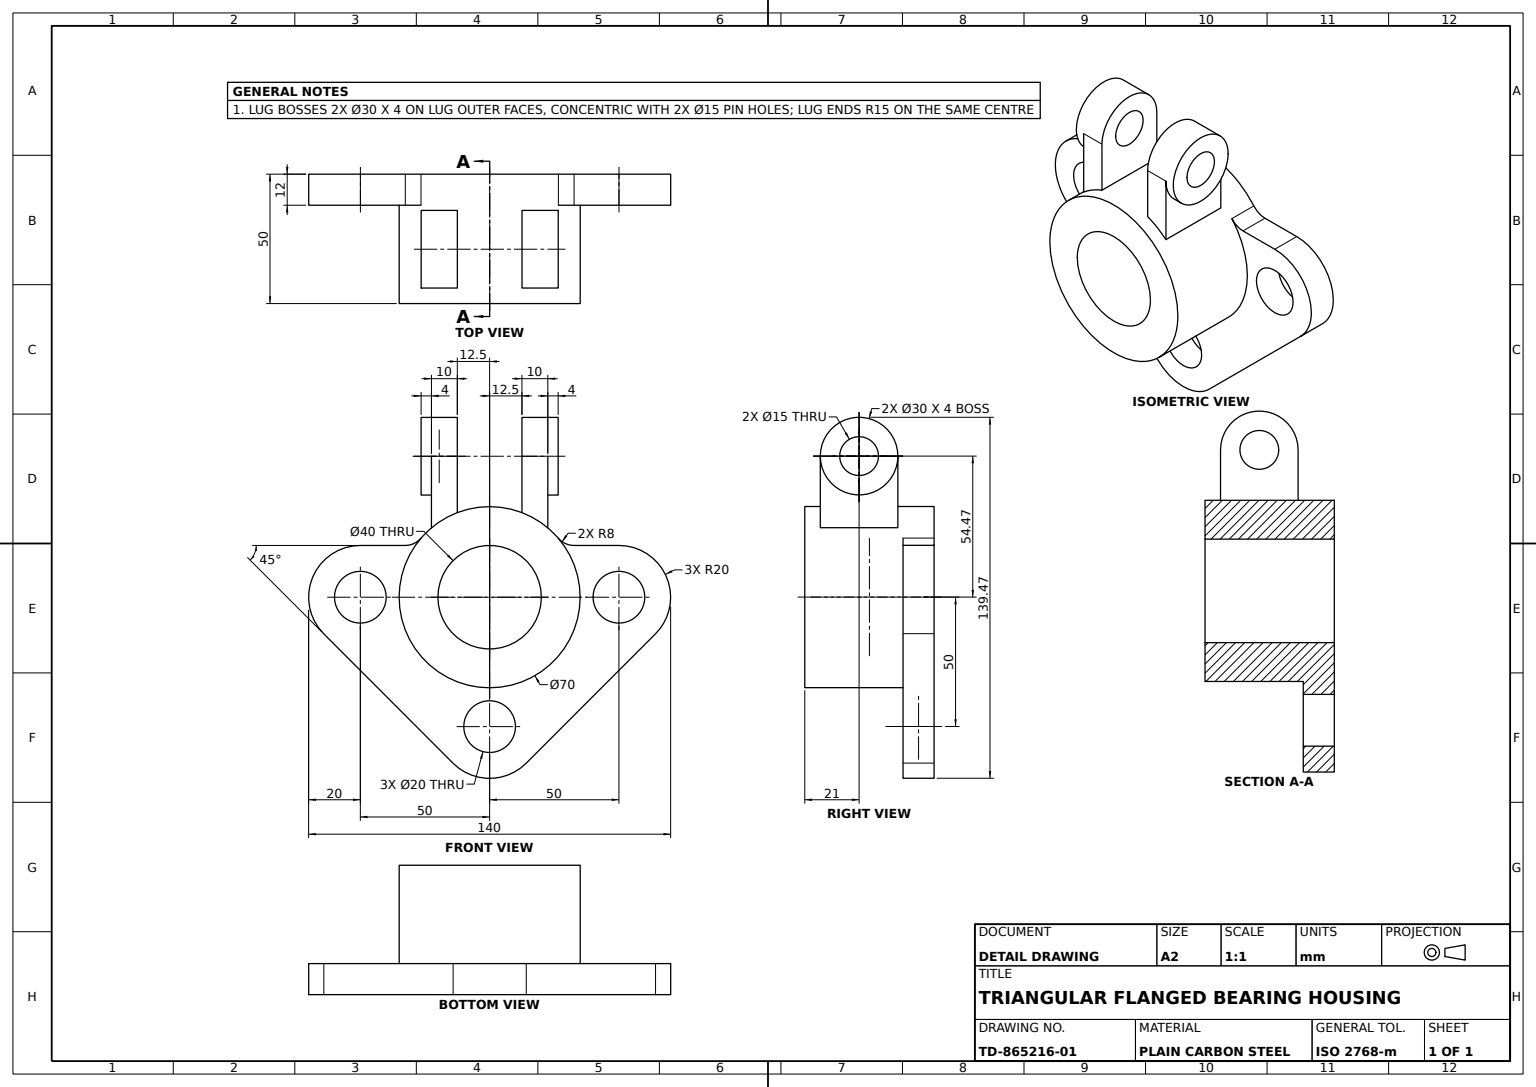
SolidWorks part; units mm, degrees
material "Plain Carbon Steel"
ref_plane "Front Plane" through (0, 0, 0) normal (0, 0, 1) x (1, 0, 0)
ref_plane "Top Plane" through (0, 0, 0) normal (0, 1, 0) x (1, 0, 0)
ref_plane "Right Plane" through (0, 0, 0) normal (1, 0, 0) x (0, 0, -1)
sketch "Hub Sketch" plane through (0, 0, 0) normal (0, 0, 1) x (1, 0, 0)
  circle A0 centre (0, 0) radius 35
  dimension "D1" = 70
extrude "Bearing Hub" add sketch "Hub Sketch" against normal blind 50
sketch "Bore Sketch" plane through (0, 0, 0) normal (0, 0, 1) x (1, 0, 0)
  circle A0 centre (0, 0) radius 20
  dimension "D1" = 40
extrude "Bearing Bore Ø40" cut sketch "Bore Sketch" against normal through all
ref_plane "Flange Plane" through (0, 0, -38) normal (0, 0, 1) x (1, 0, 0)
sketch "Flange Profile Sketch" plane through (0, 0, -38) normal (0, 0, 1) x (1, 0, 0)
  line L0 (-50, 20) -> (-28.7228, 20)
  line L1 (50, 20) -> (28.7228, 20)
  line L2 (64.1421, -14.1421) -> (14.1421, -64.1421)
  line L3 (-64.1421, -14.1421) -> (-14.1421, -64.1421)
  arc A0 (-14.1421, -64.1421) -> (14.1421, -64.1421) centre (0, -50) ccw
  arc A1 (64.1421, -14.1421) -> (50, 20) centre (50, 0) ccw
  arc A2 (-50, 20) -> (-64.1421, -14.1421) centre (-50, 0) ccw
  arc A4 (-28.7228, 20) -> (28.7228, 20) centre (0, 0) ccw
  dimension "D1" = 40
  dimension "D3" = 40
  dimension "D4" = 40
  dimension "D10" = 35
  dimension "D2" = 50
  dimension "D5" = 50
  dimension "D6" = 50
  dimension "D7" = 50
  dimension "D8" = 50
  dimension "D9" = 50
  dimension "D11" = 28.7228
  dimension "D12" = 21.2772
extrude "Mounting Flange" add sketch "Flange Profile Sketch" against normal blind 12
fillet "Flange Fillets R8" radius 8 2 edges at (-28.7228, 20, -44) (28.7228, 20, -44)
sketch "Flange Holes Sketch" plane through (0, 0, -38) normal (0, 0, 1) x (1, 0, 0)
  circle A0 centre (50, 0) radius 10
  circle A1 centre (0, -50) radius 10
  circle A2 centre (-50, 0) radius 10
  dimension "D1" = 20
  dimension "D2" = 20
  dimension "D3" = 20
extrude "Flange Mounting Holes Ø20" cut sketch "Flange Holes Sketch" against normal blind 12
ref_plane "Lug 1 Plane" through (12.5, 0, 0) normal (1, 0, 0) x (0, 0, -1)
sketch "Lug 1 Profile Sketch" plane through (12.5, 0, 0) normal (1, 0, 0) x (0, 0, -1)
  line L0 (6, 54.4714) -> (6, 26.4714)
  line L1 (6, 26.4714) -> (36, 26.4714)
  line L2 (36, 26.4714) -> (36, 54.4714)
  arc A0 (36, 54.4714) -> (6, 54.4714) centre (21, 54.4714) ccw
  dimension "D1" = 30
  dimension "D2" = 21
  dimension "D3" = 28
  dimension "D4" = 54.4714
extrude "Clevis Lug 1" add sketch "Lug 1 Profile Sketch" along normal blind 10
sketch "Lug 1 Boss Sketch" plane through (22.5, 0, 0) normal (1, 0, 0) x (0, 0, -1)
  circle A0 centre (21, 54.4714) radius 15
  dimension "D1" = 30
extrude "Lug 1 Boss Ø30" add sketch "Lug 1 Boss Sketch" along normal blind 4
ref_plane "Lug 2 Plane" through (-12.5, 0, 0) normal (1, 0, 0) x (0, 0, -1)
sketch "Lug 2 Profile Sketch" plane through (-12.5, 0, 0) normal (1, 0, 0) x (0, 0, -1)
  line L0 (36, 54.4714) -> (36, 26.4714)
  line L1 (36, 26.4714) -> (6, 26.4714)
  line L2 (6, 26.4714) -> (6, 54.4714)
  arc A0 (36, 54.4714) -> (6, 54.4714) centre (21, 54.4714) ccw
  dimension "D1" = 28
extrude "Clevis Lug 2" add sketch "Lug 2 Profile Sketch" against normal blind 10
sketch "Lug 2 Boss Sketch" plane through (-22.5, 0, 0) normal (-1, 0, 0) x (0, 0, 1)
  circle A0 centre (-21, 54.4714) radius 15
  dimension "D1" = 30
extrude "Lug 2 Boss Ø30" add sketch "Lug 2 Boss Sketch" along normal blind 4
sketch "Pin Hole Sketch" plane through (26.5, 0, 0) normal (1, 0, 0) x (0, 0, -1)
  circle A0 centre (21, 54.4714) radius 7.5
  dimension "D1" = 15
extrude "Lug Pin Hole Ø15" cut sketch "Pin Hole Sketch" against normal through all
